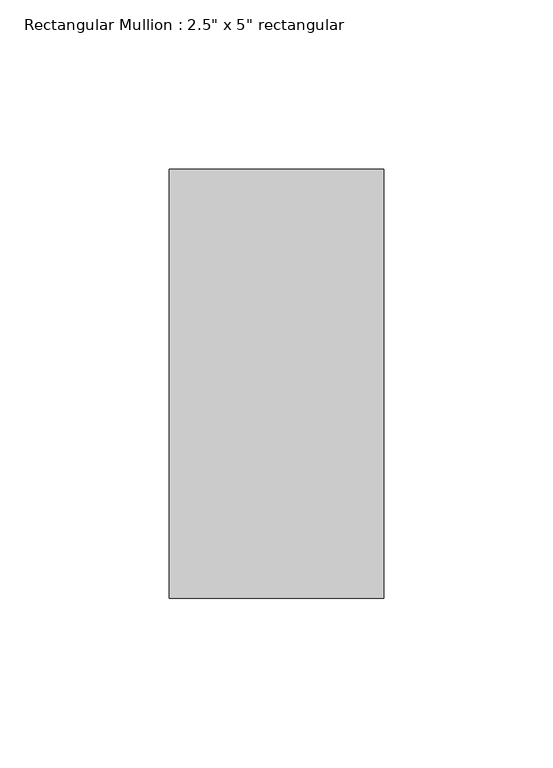
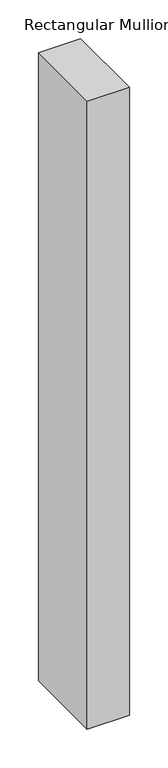
"""IFC4 building model written with IfcOpenShell, lengths in millimetres: member geometry."""

from ifc_helpers import new_model, si_unit, frame, origin, place, context, project, spatial, polyline, outline, extrude, source, transform, mapped, element, save


def member_a1cc4565(model_context):
    return source(origin(), model_context, "Body", "SweptSolid", [
        extrude(outline(polyline([(0.0, 63.5), (0.0, -63.5), (-63.5, -63.5), (-63.5, 63.5), (0.0, 63.5)])), frame((0.0, 0.0, -995.2680153), z_axis=(0.0, 0.0, 1.0), x_axis=(1.0, 0.0, 0.0)), (0.0, 0.0, 1.0), 995.2680153),
    ])


if __name__ == "__main__":
    model = new_model("IFC4")
    model_context = context("Model", 3, world=origin())
    ifc_project = project(units=[si_unit("LENGTHUNIT", "METRE", prefix="MILLI")], contexts=[model_context])
    site = spatial("IfcSite", under=ifc_project)
    building = spatial("IfcBuilding", under=site)
    placement = place(None, origin())
    member_shape = member_a1cc4565(model_context)
    element("IfcMember", 1, ObjectType="Rectangular Mullion : 2.5\" x 5\" rectangular", at=placement, inside=building, context=model_context, shape_type="MappedRepresentation", body=[
        mapped(member_shape, transform((0.0, 0.0, 0.0), x_axis=(1.0, 0.0, 0.0), y_axis=(0.0, 1.0, 0.0), z_axis=(0.0, 0.0, 1.0))),
    ])
    save(model, "model.ifc")

# Revit data of these elements
# Type "Rectangular Mullion : 2.5\" x 5\" rectangular"
#   built-in parameter 1007304 = 0.416667 (stored number, unit not read)
#   built-in parameter 1007301 = 0.104167 (stored number, unit not read)
#   built-in parameter 1007300 = 0.104167 (stored number, unit not read)
# Element 1 (IfcMember, "Rectangular Mullion : 2.5\" x 5\" rectangular")
#   Materials on its faces: "Aluminum"
# Materials
#   "Aluminum": class "Metal", colour RGB 247 247 247, transparency 0, Description = "Aluminum 6061", Cost = 0
